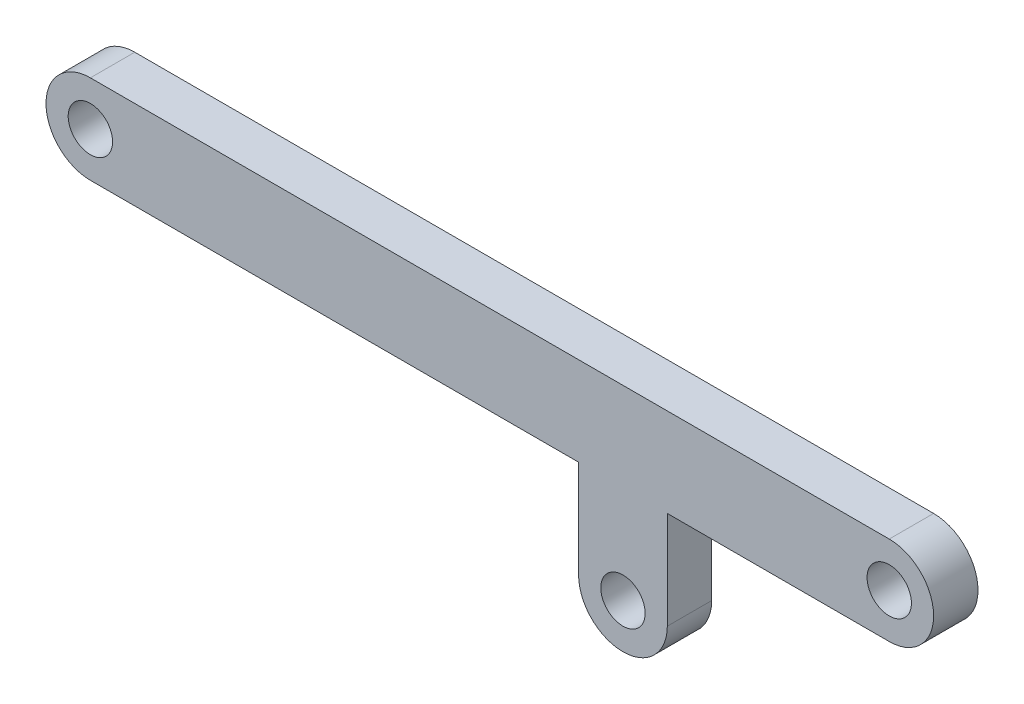
ISO-10303-21;
HEADER;
FILE_DESCRIPTION(('STEP AP214'),'2;1');
FILE_NAME('part.step','',(''),(''),'','','');
FILE_SCHEMA(('AUTOMOTIVE_DESIGN { 1 0 10303 214 1 1 1 1 }'));
ENDSEC;
DATA;
#1=APPLICATION_CONTEXT('core data for automotive mechanical design processes');
#2=APPLICATION_PROTOCOL_DEFINITION('international standard','automotive_design',2000,#1);
#3=PRODUCT_CONTEXT('',#1,'mechanical');
#4=PRODUCT('Part','Part','',(#3));
#5=PRODUCT_RELATED_PRODUCT_CATEGORY('part','',(#4));
#6=PRODUCT_DEFINITION_FORMATION('','',#4);
#7=PRODUCT_DEFINITION_CONTEXT('part definition',#1,'design');
#8=PRODUCT_DEFINITION('design','',#6,#7);
#9=PRODUCT_DEFINITION_SHAPE('','',#8);
#10=(LENGTH_UNIT() NAMED_UNIT(*) SI_UNIT(.MILLI.,.METRE.));
#11=(NAMED_UNIT(*) PLANE_ANGLE_UNIT() SI_UNIT($,.RADIAN.));
#12=(NAMED_UNIT(*) SI_UNIT($,.STERADIAN.) SOLID_ANGLE_UNIT());
#13=UNCERTAINTY_MEASURE_WITH_UNIT(LENGTH_MEASURE(1.E-05),#10,'distance_accuracy_value','');
#14=(GEOMETRIC_REPRESENTATION_CONTEXT(3) GLOBAL_UNCERTAINTY_ASSIGNED_CONTEXT((#13)) GLOBAL_UNIT_ASSIGNED_CONTEXT((#10,
#11,#12)) REPRESENTATION_CONTEXT('',''));
#15=CARTESIAN_POINT('',(0.,0.,0.));
#16=DIRECTION('',(0.,0.,1.));
#17=DIRECTION('',(1.,0.,0.));
#18=AXIS2_PLACEMENT_3D('',#15,#16,#17);
#19=CARTESIAN_POINT('',(0.,5.00000000000001,2.5));
#20=DIRECTION('',(0.,-1.,0.));
#21=DIRECTION('',(1.,0.,0.));
#22=AXIS2_PLACEMENT_3D('',#19,#20,#21);
#23=PLANE('',#22);
#24=DIRECTION('',(-1.,0.,0.));
#25=VECTOR('',#24,1.);
#26=CARTESIAN_POINT('',(0.,5.00000000000001,-2.5));
#27=LINE('',#26,#25);
#28=CARTESIAN_POINT('',(45.,5.00000000000002,-2.5));
#29=VERTEX_POINT('',#28);
#30=CARTESIAN_POINT('',(-45.,4.99999999999999,-2.5));
#31=VERTEX_POINT('',#30);
#32=EDGE_CURVE('E148',#29,#31,#27,.T.);
#33=ORIENTED_EDGE('',*,*,#32,.T.);
#34=DIRECTION('',(0.,0.,-1.));
#35=VECTOR('',#34,1.);
#36=CARTESIAN_POINT('',(-45.,4.99999999999999,2.5));
#37=LINE('',#36,#35);
#38=CARTESIAN_POINT('',(-45.,4.99999999999999,2.5));
#39=VERTEX_POINT('',#38);
#40=EDGE_CURVE('E11',#39,#31,#37,.T.);
#41=ORIENTED_EDGE('',*,*,#40,.F.);
#42=DIRECTION('',(-1.,0.,0.));
#43=VECTOR('',#42,1.);
#44=CARTESIAN_POINT('',(0.,5.00000000000001,2.5));
#45=LINE('',#44,#43);
#46=CARTESIAN_POINT('',(45.,5.00000000000002,2.5));
#47=VERTEX_POINT('',#46);
#48=EDGE_CURVE('E201',#47,#39,#45,.T.);
#49=ORIENTED_EDGE('',*,*,#48,.F.);
#50=DIRECTION('',(0.,0.,-1.));
#51=VECTOR('',#50,1.);
#52=CARTESIAN_POINT('',(45.,5.00000000000002,2.5));
#53=LINE('',#52,#51);
#54=EDGE_CURVE('E142',#47,#29,#53,.T.);
#55=ORIENTED_EDGE('',*,*,#54,.T.);
#56=EDGE_LOOP('',(#33,#41,#49,#55));
#57=FACE_BOUND('',#56,.T.);
#58=ADVANCED_FACE('F41',(#57),#23,.F.);
#59=CARTESIAN_POINT('',(-45.,0.,2.5));
#60=DIRECTION('',(0.,0.,-1.));
#61=DIRECTION('',(-1.,0.,0.));
#62=AXIS2_PLACEMENT_3D('',#59,#60,#61);
#63=CYLINDRICAL_SURFACE('',#62,5.);
#64=CARTESIAN_POINT('',(-45.,0.,-2.5));
#65=DIRECTION('',(0.,0.,1.));
#66=DIRECTION('',(1.,0.,0.));
#67=AXIS2_PLACEMENT_3D('',#64,#65,#66);
#68=CIRCLE('',#67,5.);
#69=CARTESIAN_POINT('',(-45.,-5.00000000000001,-2.5));
#70=VERTEX_POINT('',#69);
#71=EDGE_CURVE('E149',#31,#70,#68,.T.);
#72=ORIENTED_EDGE('',*,*,#71,.T.);
#73=DIRECTION('',(0.,0.,-1.));
#74=VECTOR('',#73,1.);
#75=CARTESIAN_POINT('',(-45.,-5.00000000000001,2.5));
#76=LINE('',#75,#74);
#77=CARTESIAN_POINT('',(-45.,-5.00000000000001,2.5));
#78=VERTEX_POINT('',#77);
#79=EDGE_CURVE('E49',#78,#70,#76,.T.);
#80=ORIENTED_EDGE('',*,*,#79,.F.);
#81=CARTESIAN_POINT('',(-45.,0.,2.5));
#82=DIRECTION('',(0.,0.,1.));
#83=DIRECTION('',(1.,0.,0.));
#84=AXIS2_PLACEMENT_3D('',#81,#82,#83);
#85=CIRCLE('',#84,5.);
#86=EDGE_CURVE('E100',#39,#78,#85,.T.);
#87=ORIENTED_EDGE('',*,*,#86,.F.);
#88=ORIENTED_EDGE('',*,*,#40,.T.);
#89=EDGE_LOOP('',(#72,#80,#87,#88));
#90=FACE_BOUND('',#89,.T.);
#91=ADVANCED_FACE('F184',(#90),#63,.T.);
#92=CARTESIAN_POINT('',(0.,-5.,2.5));
#93=DIRECTION('',(0.,-1.,0.));
#94=DIRECTION('',(1.,0.,0.));
#95=AXIS2_PLACEMENT_3D('',#92,#93,#94);
#96=PLANE('',#95);
#97=DIRECTION('',(-1.,0.,0.));
#98=VECTOR('',#97,1.);
#99=CARTESIAN_POINT('',(0.,-5.,-2.5));
#100=LINE('',#99,#98);
#101=CARTESIAN_POINT('',(10.,-4.99999999999999,-2.5));
#102=VERTEX_POINT('',#101);
#103=EDGE_CURVE('E155',#102,#70,#100,.T.);
#104=ORIENTED_EDGE('',*,*,#103,.F.);
#105=DIRECTION('',(0.,0.,-1.));
#106=VECTOR('',#105,1.);
#107=CARTESIAN_POINT('',(10.,-4.99999999999999,2.5));
#108=LINE('',#107,#106);
#109=CARTESIAN_POINT('',(10.,-4.99999999999999,2.5));
#110=VERTEX_POINT('',#109);
#111=EDGE_CURVE('E176',#110,#102,#108,.T.);
#112=ORIENTED_EDGE('',*,*,#111,.F.);
#113=DIRECTION('',(-1.,0.,0.));
#114=VECTOR('',#113,1.);
#115=CARTESIAN_POINT('',(0.,-5.,2.5));
#116=LINE('',#115,#114);
#117=EDGE_CURVE('E181',#110,#78,#116,.T.);
#118=ORIENTED_EDGE('',*,*,#117,.T.);
#119=ORIENTED_EDGE('',*,*,#79,.T.);
#120=EDGE_LOOP('',(#104,#112,#118,#119));
#121=FACE_BOUND('',#120,.T.);
#122=ADVANCED_FACE('F182',(#121),#96,.T.);
#123=CARTESIAN_POINT('',(10.,0.,2.5));
#124=DIRECTION('',(1.,0.,0.));
#125=DIRECTION('',(0.,1.,0.));
#126=AXIS2_PLACEMENT_3D('',#123,#124,#125);
#127=PLANE('',#126);
#128=DIRECTION('',(0.,-1.,0.));
#129=VECTOR('',#128,1.);
#130=CARTESIAN_POINT('',(10.,0.,-2.5));
#131=LINE('',#130,#129);
#132=CARTESIAN_POINT('',(10.,-16.,-2.5));
#133=VERTEX_POINT('',#132);
#134=EDGE_CURVE('E154',#102,#133,#131,.T.);
#135=ORIENTED_EDGE('',*,*,#134,.T.);
#136=DIRECTION('',(0.,0.,-1.));
#137=VECTOR('',#136,1.);
#138=CARTESIAN_POINT('',(10.,-16.,2.5));
#139=LINE('',#138,#137);
#140=CARTESIAN_POINT('',(10.,-16.,2.5));
#141=VERTEX_POINT('',#140);
#142=EDGE_CURVE('E171',#141,#133,#139,.T.);
#143=ORIENTED_EDGE('',*,*,#142,.F.);
#144=DIRECTION('',(0.,-1.,0.));
#145=VECTOR('',#144,1.);
#146=CARTESIAN_POINT('',(10.,0.,2.5));
#147=LINE('',#146,#145);
#148=EDGE_CURVE('E196',#110,#141,#147,.T.);
#149=ORIENTED_EDGE('',*,*,#148,.F.);
#150=ORIENTED_EDGE('',*,*,#111,.T.);
#151=EDGE_LOOP('',(#135,#143,#149,#150));
#152=FACE_BOUND('',#151,.T.);
#153=ADVANCED_FACE('F193',(#152),#127,.F.);
#154=CARTESIAN_POINT('',(15.,-16.,2.5));
#155=DIRECTION('',(0.,0.,-1.));
#156=DIRECTION('',(-1.,0.,0.));
#157=AXIS2_PLACEMENT_3D('',#154,#155,#156);
#158=CYLINDRICAL_SURFACE('',#157,5.);
#159=CARTESIAN_POINT('',(15.,-16.,-2.5));
#160=DIRECTION('',(0.,0.,1.));
#161=DIRECTION('',(1.,0.,0.));
#162=AXIS2_PLACEMENT_3D('',#159,#160,#161);
#163=CIRCLE('',#162,5.);
#164=CARTESIAN_POINT('',(20.,-16.,-2.5));
#165=VERTEX_POINT('',#164);
#166=EDGE_CURVE('E160',#133,#165,#163,.T.);
#167=ORIENTED_EDGE('',*,*,#166,.T.);
#168=DIRECTION('',(0.,0.,-1.));
#169=VECTOR('',#168,1.);
#170=CARTESIAN_POINT('',(20.,-16.,2.5));
#171=LINE('',#170,#169);
#172=CARTESIAN_POINT('',(20.,-16.,2.5));
#173=VERTEX_POINT('',#172);
#174=EDGE_CURVE('E121',#173,#165,#171,.T.);
#175=ORIENTED_EDGE('',*,*,#174,.F.);
#176=CARTESIAN_POINT('',(15.,-16.,2.5));
#177=DIRECTION('',(0.,0.,1.));
#178=DIRECTION('',(1.,0.,0.));
#179=AXIS2_PLACEMENT_3D('',#176,#177,#178);
#180=CIRCLE('',#179,5.);
#181=EDGE_CURVE('E126',#141,#173,#180,.T.);
#182=ORIENTED_EDGE('',*,*,#181,.F.);
#183=ORIENTED_EDGE('',*,*,#142,.T.);
#184=EDGE_LOOP('',(#167,#175,#182,#183));
#185=FACE_BOUND('',#184,.T.);
#186=ADVANCED_FACE('F197',(#185),#158,.T.);
#187=CARTESIAN_POINT('',(20.,0.,2.5));
#188=DIRECTION('',(1.,0.,0.));
#189=DIRECTION('',(0.,1.,0.));
#190=AXIS2_PLACEMENT_3D('',#187,#188,#189);
#191=PLANE('',#190);
#192=DIRECTION('',(0.,-1.,0.));
#193=VECTOR('',#192,1.);
#194=CARTESIAN_POINT('',(20.,0.,-2.5));
#195=LINE('',#194,#193);
#196=CARTESIAN_POINT('',(20.,-4.99999999999999,-2.5));
#197=VERTEX_POINT('',#196);
#198=EDGE_CURVE('E120',#197,#165,#195,.T.);
#199=ORIENTED_EDGE('',*,*,#198,.F.);
#200=DIRECTION('',(0.,0.,-1.));
#201=VECTOR('',#200,1.);
#202=CARTESIAN_POINT('',(20.,-4.99999999999999,2.5));
#203=LINE('',#202,#201);
#204=CARTESIAN_POINT('',(20.,-4.99999999999999,2.5));
#205=VERTEX_POINT('',#204);
#206=EDGE_CURVE('E115',#205,#197,#203,.T.);
#207=ORIENTED_EDGE('',*,*,#206,.F.);
#208=DIRECTION('',(0.,-1.,0.));
#209=VECTOR('',#208,1.);
#210=CARTESIAN_POINT('',(20.,0.,2.5));
#211=LINE('',#210,#209);
#212=EDGE_CURVE('E113',#205,#173,#211,.T.);
#213=ORIENTED_EDGE('',*,*,#212,.T.);
#214=ORIENTED_EDGE('',*,*,#174,.T.);
#215=EDGE_LOOP('',(#199,#207,#213,#214));
#216=FACE_BOUND('',#215,.T.);
#217=ADVANCED_FACE('F111',(#216),#191,.T.);
#218=CARTESIAN_POINT('',(0.,-5.,2.5));
#219=DIRECTION('',(0.,-1.,0.));
#220=DIRECTION('',(1.,0.,0.));
#221=AXIS2_PLACEMENT_3D('',#218,#219,#220);
#222=PLANE('',#221);
#223=DIRECTION('',(-1.,0.,0.));
#224=VECTOR('',#223,1.);
#225=CARTESIAN_POINT('',(0.,-5.,-2.5));
#226=LINE('',#225,#224);
#227=CARTESIAN_POINT('',(45.,-4.99999999999998,-2.5));
#228=VERTEX_POINT('',#227);
#229=EDGE_CURVE('E161',#228,#197,#226,.T.);
#230=ORIENTED_EDGE('',*,*,#229,.F.);
#231=DIRECTION('',(0.,0.,-1.));
#232=VECTOR('',#231,1.);
#233=CARTESIAN_POINT('',(45.,-4.99999999999998,2.5));
#234=LINE('',#233,#232);
#235=CARTESIAN_POINT('',(45.,-4.99999999999998,2.5));
#236=VERTEX_POINT('',#235);
#237=EDGE_CURVE('E88',#236,#228,#234,.T.);
#238=ORIENTED_EDGE('',*,*,#237,.F.);
#239=DIRECTION('',(-1.,0.,0.));
#240=VECTOR('',#239,1.);
#241=CARTESIAN_POINT('',(0.,-5.,2.5));
#242=LINE('',#241,#240);
#243=EDGE_CURVE('E127',#236,#205,#242,.T.);
#244=ORIENTED_EDGE('',*,*,#243,.T.);
#245=ORIENTED_EDGE('',*,*,#206,.T.);
#246=EDGE_LOOP('',(#230,#238,#244,#245));
#247=FACE_BOUND('',#246,.T.);
#248=ADVANCED_FACE('F132',(#247),#222,.T.);
#249=CARTESIAN_POINT('',(45.,0.,2.5));
#250=DIRECTION('',(0.,0.,-1.));
#251=DIRECTION('',(-1.,0.,0.));
#252=AXIS2_PLACEMENT_3D('',#249,#250,#251);
#253=CYLINDRICAL_SURFACE('',#252,2.5);
#254=CARTESIAN_POINT('',(45.,0.,2.5));
#255=DIRECTION('',(0.,0.,1.));
#256=DIRECTION('',(1.,0.,0.));
#257=AXIS2_PLACEMENT_3D('',#254,#255,#256);
#258=CIRCLE('',#257,2.5);
#259=CARTESIAN_POINT('',(47.5,0.,2.5));
#260=VERTEX_POINT('',#259);
#261=EDGE_CURVE('E134',#260,#260,#258,.T.);
#262=ORIENTED_EDGE('',*,*,#261,.T.);
#263=EDGE_LOOP('',(#262));
#264=FACE_BOUND('',#263,.T.);
#265=CARTESIAN_POINT('',(45.,0.,-2.5));
#266=DIRECTION('',(0.,0.,1.));
#267=DIRECTION('',(1.,0.,0.));
#268=AXIS2_PLACEMENT_3D('',#265,#266,#267);
#269=CIRCLE('',#268,2.5);
#270=CARTESIAN_POINT('',(47.5,0.,-2.5));
#271=VERTEX_POINT('',#270);
#272=EDGE_CURVE('E163',#271,#271,#269,.T.);
#273=ORIENTED_EDGE('',*,*,#272,.F.);
#274=EDGE_LOOP('',(#273));
#275=FACE_BOUND('',#274,.T.);
#276=ADVANCED_FACE('F236',(#264,#275),#253,.F.);
#277=CARTESIAN_POINT('',(45.,0.,2.5));
#278=DIRECTION('',(0.,0.,-1.));
#279=DIRECTION('',(-1.,0.,0.));
#280=AXIS2_PLACEMENT_3D('',#277,#278,#279);
#281=CYLINDRICAL_SURFACE('',#280,5.);
#282=CARTESIAN_POINT('',(45.,0.,-2.5));
#283=DIRECTION('',(0.,0.,1.));
#284=DIRECTION('',(1.,0.,0.));
#285=AXIS2_PLACEMENT_3D('',#282,#283,#284);
#286=CIRCLE('',#285,5.);
#287=EDGE_CURVE('E90',#228,#29,#286,.T.);
#288=ORIENTED_EDGE('',*,*,#287,.T.);
#289=ORIENTED_EDGE('',*,*,#54,.F.);
#290=CARTESIAN_POINT('',(45.,0.,2.5));
#291=DIRECTION('',(0.,0.,1.));
#292=DIRECTION('',(1.,0.,0.));
#293=AXIS2_PLACEMENT_3D('',#290,#291,#292);
#294=CIRCLE('',#293,5.);
#295=EDGE_CURVE('E59',#236,#47,#294,.T.);
#296=ORIENTED_EDGE('',*,*,#295,.F.);
#297=ORIENTED_EDGE('',*,*,#237,.T.);
#298=EDGE_LOOP('',(#288,#289,#296,#297));
#299=FACE_BOUND('',#298,.T.);
#300=ADVANCED_FACE('F239',(#299),#281,.T.);
#301=CARTESIAN_POINT('',(-45.,0.,2.5));
#302=DIRECTION('',(0.,0.,-1.));
#303=DIRECTION('',(-1.,0.,0.));
#304=AXIS2_PLACEMENT_3D('',#301,#302,#303);
#305=CYLINDRICAL_SURFACE('',#304,2.5);
#306=CARTESIAN_POINT('',(-45.,0.,2.5));
#307=DIRECTION('',(0.,0.,1.));
#308=DIRECTION('',(1.,0.,0.));
#309=AXIS2_PLACEMENT_3D('',#306,#307,#308);
#310=CIRCLE('',#309,2.5);
#311=CARTESIAN_POINT('',(-42.5,0.,2.5));
#312=VERTEX_POINT('',#311);
#313=EDGE_CURVE('E168',#312,#312,#310,.T.);
#314=ORIENTED_EDGE('',*,*,#313,.T.);
#315=EDGE_LOOP('',(#314));
#316=FACE_BOUND('',#315,.T.);
#317=CARTESIAN_POINT('',(-45.,0.,-2.5));
#318=DIRECTION('',(0.,0.,1.));
#319=DIRECTION('',(1.,0.,0.));
#320=AXIS2_PLACEMENT_3D('',#317,#318,#319);
#321=CIRCLE('',#320,2.5);
#322=CARTESIAN_POINT('',(-42.5,0.,-2.5));
#323=VERTEX_POINT('',#322);
#324=EDGE_CURVE('E141',#323,#323,#321,.T.);
#325=ORIENTED_EDGE('',*,*,#324,.F.);
#326=EDGE_LOOP('',(#325));
#327=FACE_BOUND('',#326,.T.);
#328=ADVANCED_FACE('F43',(#316,#327),#305,.F.);
#329=CARTESIAN_POINT('',(15.,-16.,2.5));
#330=DIRECTION('',(0.,0.,-1.));
#331=DIRECTION('',(-1.,0.,0.));
#332=AXIS2_PLACEMENT_3D('',#329,#330,#331);
#333=CYLINDRICAL_SURFACE('',#332,2.5);
#334=CARTESIAN_POINT('',(15.,-16.,2.5));
#335=DIRECTION('',(0.,0.,1.));
#336=DIRECTION('',(1.,0.,0.));
#337=AXIS2_PLACEMENT_3D('',#334,#335,#336);
#338=CIRCLE('',#337,2.5);
#339=CARTESIAN_POINT('',(17.5,-16.,2.5));
#340=VERTEX_POINT('',#339);
#341=EDGE_CURVE('E138',#340,#340,#338,.T.);
#342=ORIENTED_EDGE('',*,*,#341,.T.);
#343=EDGE_LOOP('',(#342));
#344=FACE_BOUND('',#343,.T.);
#345=CARTESIAN_POINT('',(15.,-16.,-2.5));
#346=DIRECTION('',(0.,0.,1.));
#347=DIRECTION('',(1.,0.,0.));
#348=AXIS2_PLACEMENT_3D('',#345,#346,#347);
#349=CIRCLE('',#348,2.5);
#350=CARTESIAN_POINT('',(17.5,-16.,-2.5));
#351=VERTEX_POINT('',#350);
#352=EDGE_CURVE('E170',#351,#351,#349,.T.);
#353=ORIENTED_EDGE('',*,*,#352,.F.);
#354=EDGE_LOOP('',(#353));
#355=FACE_BOUND('',#354,.T.);
#356=ADVANCED_FACE('F211',(#344,#355),#333,.F.);
#357=CARTESIAN_POINT('',(0.,0.,2.5));
#358=DIRECTION('',(0.,0.,1.));
#359=DIRECTION('',(1.,0.,0.));
#360=AXIS2_PLACEMENT_3D('',#357,#358,#359);
#361=PLANE('',#360);
#362=ORIENTED_EDGE('',*,*,#313,.F.);
#363=EDGE_LOOP('',(#362));
#364=FACE_BOUND('',#363,.T.);
#365=ORIENTED_EDGE('',*,*,#48,.T.);
#366=ORIENTED_EDGE('',*,*,#86,.T.);
#367=ORIENTED_EDGE('',*,*,#117,.F.);
#368=ORIENTED_EDGE('',*,*,#148,.T.);
#369=ORIENTED_EDGE('',*,*,#181,.T.);
#370=ORIENTED_EDGE('',*,*,#212,.F.);
#371=ORIENTED_EDGE('',*,*,#243,.F.);
#372=ORIENTED_EDGE('',*,*,#295,.T.);
#373=EDGE_LOOP('',(#365,#366,#367,#368,#369,#370,#371,#372));
#374=FACE_BOUND('',#373,.T.);
#375=ORIENTED_EDGE('',*,*,#261,.F.);
#376=EDGE_LOOP('',(#375));
#377=FACE_BOUND('',#376,.T.);
#378=ORIENTED_EDGE('',*,*,#341,.F.);
#379=EDGE_LOOP('',(#378));
#380=FACE_BOUND('',#379,.T.);
#381=ADVANCED_FACE('F123',(#364,#374,#377,#380),#361,.T.);
#382=CARTESIAN_POINT('',(0.,0.,-2.5));
#383=DIRECTION('',(0.,0.,1.));
#384=DIRECTION('',(1.,0.,0.));
#385=AXIS2_PLACEMENT_3D('',#382,#383,#384);
#386=PLANE('',#385);
#387=ORIENTED_EDGE('',*,*,#324,.T.);
#388=EDGE_LOOP('',(#387));
#389=FACE_BOUND('',#388,.T.);
#390=ORIENTED_EDGE('',*,*,#32,.F.);
#391=ORIENTED_EDGE('',*,*,#287,.F.);
#392=ORIENTED_EDGE('',*,*,#229,.T.);
#393=ORIENTED_EDGE('',*,*,#198,.T.);
#394=ORIENTED_EDGE('',*,*,#166,.F.);
#395=ORIENTED_EDGE('',*,*,#134,.F.);
#396=ORIENTED_EDGE('',*,*,#103,.T.);
#397=ORIENTED_EDGE('',*,*,#71,.F.);
#398=EDGE_LOOP('',(#390,#391,#392,#393,#394,#395,#396,#397));
#399=FACE_BOUND('',#398,.T.);
#400=ORIENTED_EDGE('',*,*,#272,.T.);
#401=EDGE_LOOP('',(#400));
#402=FACE_BOUND('',#401,.T.);
#403=ORIENTED_EDGE('',*,*,#352,.T.);
#404=EDGE_LOOP('',(#403));
#405=FACE_BOUND('',#404,.T.);
#406=ADVANCED_FACE('F186',(#389,#399,#402,#405),#386,.F.);
#407=CLOSED_SHELL('',(#58,#91,#122,#153,#186,#217,#248,#276,#300,#328,#356,#381,#406));
#408=MANIFOLD_SOLID_BREP('B2',#407);
#409=ADVANCED_BREP_SHAPE_REPRESENTATION('',(#18,#408),#14);
#410=SHAPE_DEFINITION_REPRESENTATION(#9,#409);
ENDSEC;
END-ISO-10303-21;
